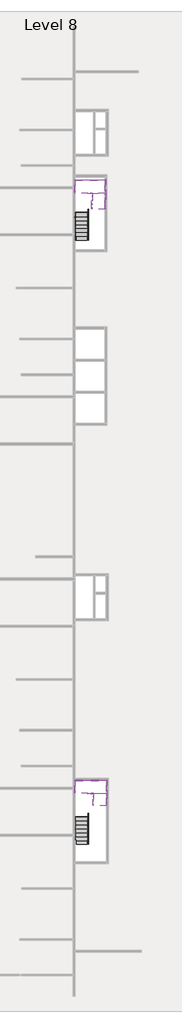
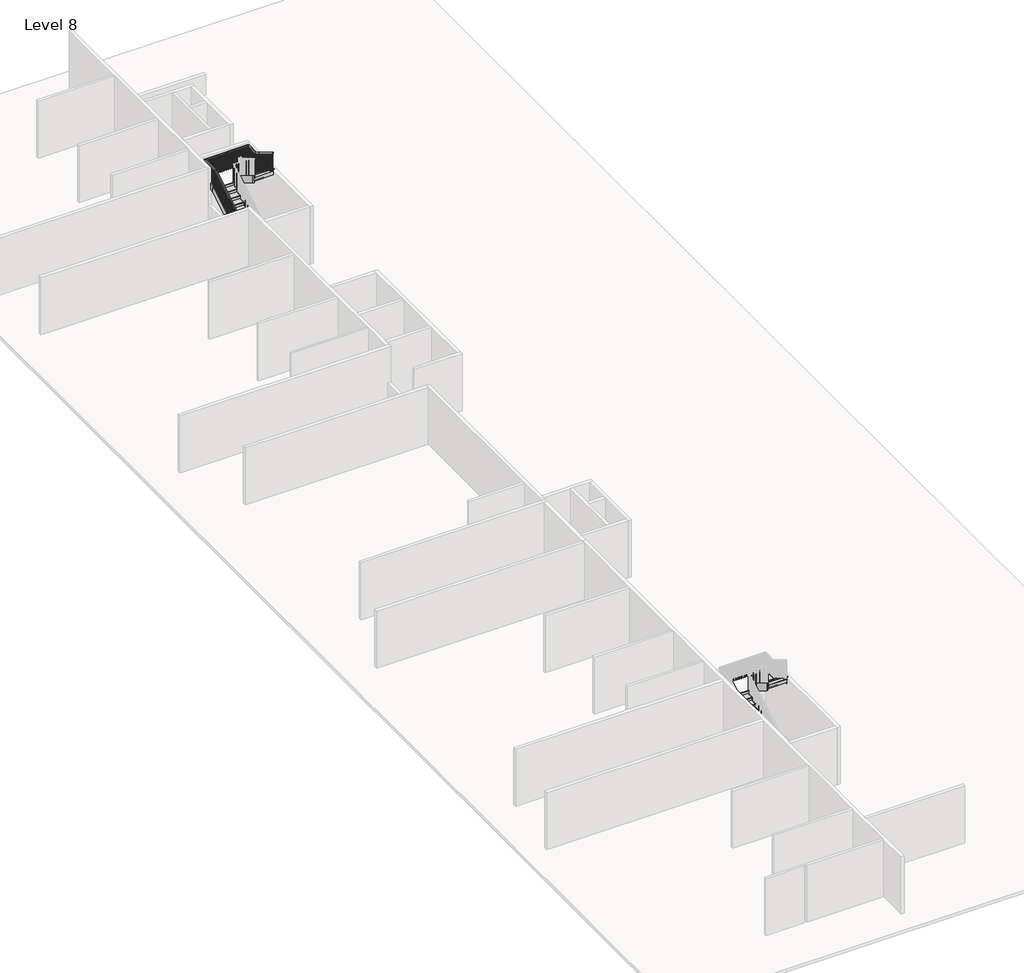
# One storey, part 8 of 8: 16 members, 4 stair flights, 2 slabs, 1 railing.
"""IFC4 building model written with IfcOpenShell, lengths in millimetres."""

from ifc_helpers import new_model, si_unit, frame, origin, place, context, project, spatial, polyline, outline, extrude, faceted_brep, transform, mapped, element, save
from components import non_monolithic_landing_8e40c115, non_monolithic_landing_da8bd63b, stair_flight_80be26fe, stair_flight_738362f5, stair_flight_d970984e, stair_flight_6e3cd39c

model = new_model("IFC4")

# Units and contexts
model_context = context("Model", 3, world=origin())
ifc_project = project(units=[si_unit("LENGTHUNIT", "METRE", prefix="MILLI")], contexts=[model_context])

# Site, building, storey
site = spatial("IfcSite", under=ifc_project)
building = spatial("IfcBuilding", under=site)
storey = spatial("IfcBuildingStorey", under=building, Name="Level 8", Elevation=46570.6172466)

# Members
placement = place(None, origin())
element("IfcMember", 1, ObjectType="Stringer - 2\" Width", at=placement, inside=storey, context=model_context, shape_type="SweptSolid", body=[
    extrude(outline(polyline([(-23154.3851539, 46570.6172466), (-23154.3851539, 46782.7317586), (-19467.0440987, 49017.4839133), (-19381.8896422, 48712.6839133), (-22916.2996422, 46570.6172466), (-23154.3851539, 46570.6172466)])), frame((-3668.2415084, 0.0, 0.0), z_axis=(1.0, 0.0, 0.0), x_axis=(0.0, 1.0, 0.0)), (0.0, 0.0, 1.0), 50.8),
])
element("IfcMember", 2, ObjectType="Stringer - 2\" Width", at=placement, inside=storey, context=model_context, shape_type="SweptSolid", body=[
    extrude(outline(polyline([(-23154.3851539, 46570.6172466), (-23154.3851539, 46782.7317586), (-19572.9851539, 48953.2772131), (-19572.9851539, 48596.8684516), (-22916.2996422, 46570.6172466), (-23154.3851539, 46570.6172466)])), frame((-2703.0415084, 0.0, 0.0), z_axis=(1.0, 0.0, 0.0), x_axis=(0.0, 1.0, 0.0)), (0.0, 0.0, 1.0), 50.8),
])
element("IfcMember", 3, ObjectType="Stringer - 2\" Width", at=placement, inside=storey, context=model_context, shape_type="SweptSolid", body=[
    extrude(outline(polyline([(-19297.9262092, 49017.4839133), (-19383.0806657, 48712.6839133), (-20360.3851539, 49304.9896637), (-20360.3851539, 49661.3984252), (-19297.9262092, 49017.4839133)])), frame((-1382.2415084, 0.0, 0.0), z_axis=(1.0, 0.0, 0.0), x_axis=(0.0, 1.0, 0.0)), (0.0, 0.0, 1.0), 50.8),
])
element("IfcMember", 4, ObjectType="Stringer - 2\" Width", at=placement, inside=storey, context=model_context, shape_type="SweptSolid", body=[
    extrude(outline(polyline([(-19522.1851539, 49153.3984252), (-19522.1851539, 48796.9896637), (-20360.3851539, 49304.9896637), (-20360.3851539, 49661.3984252), (-19522.1851539, 49153.3984252)])), frame((-2347.4415084, 0.0, 0.0), z_axis=(1.0, 0.0, 0.0), x_axis=(0.0, 1.0, 0.0)), (0.0, 0.0, 1.0), 50.8),
])
element("IfcMember", 5, ObjectType="Stringer - 2\" Width", at=placement, inside=storey, context=model_context, shape_type="Brep", body=[
    faceted_brep([(-1382.2415084, -19297.9262092, 49017.4839133), (-1331.4415084, -19297.9262092, 49017.4839133), (-1331.4415084, -18556.9851539, 49017.4839133), (-1382.2415084, -18607.7851539, 49017.4839133), (-1382.2415084, -19383.0806657, 48712.6839133), (-1382.2415084, -18607.7851539, 48712.6839133), (-1331.4415084, -19383.0806657, 48712.6839133), (-1331.4415084, -18556.9851539, 48712.6839133)], [[[0, 1, 2, 3]], [[4, 0, 3, 5]], [[6, 4, 5, 7]], [[1, 6, 7, 2]], [[1, 0, 4, 6]], [[2, 7, 5, 3]]]),
])
element("IfcMember", 6, ObjectType="Stringer - 2\" Width", at=placement, inside=storey, context=model_context, shape_type="SweptSolid", body=[
    extrude(outline(polyline([(-1331.4415084, -18556.9851539), (-1382.2415084, -18607.7851539), (-3617.4415084, -18607.7851539), (-3668.2415084, -18556.9851539), (-1331.4415084, -18556.9851539)])), frame((0.0, 0.0, 48712.6839133), z_axis=(0.0, 0.0, 1.0), x_axis=(1.0, 0.0, 0.0)), (0.0, 0.0, 1.0), 304.8),
])
element("IfcMember", 7, ObjectType="Stringer - 2\" Width", at=placement, inside=storey, context=model_context, shape_type="Brep", body=[
    faceted_brep([(-3617.4415084, -18607.7851539, 49017.4839133), (-3668.2415084, -18556.9851539, 49017.4839133), (-3668.2415084, -19467.0440987, 49017.4839133), (-3617.4415084, -19467.0440987, 49017.4839133), (-3617.4415084, -18607.7851539, 48712.6839133), (-3617.4415084, -19381.8896422, 48712.6839133), (-3668.2415084, -18556.9851539, 48712.6839133), (-3668.2415084, -19381.8896422, 48712.6839133)], [[[0, 1, 2, 3]], [[4, 0, 3, 5]], [[6, 4, 5, 7]], [[1, 6, 7, 2]], [[1, 0, 4, 6]], [[2, 7, 5, 3]]]),
])
element("IfcMember", 8, ObjectType="Stringer - 2\" Width", at=placement, inside=storey, context=model_context, shape_type="SweptSolid", body=[
    extrude(outline(polyline([(-2703.0415084, -19572.9851539), (-2703.0415084, -19522.1851539), (-2347.4415084, -19522.1851539), (-2347.4415084, -19572.9851539), (-2703.0415084, -19572.9851539)])), frame((0.0, 0.0, 48712.6839133), z_axis=(0.0, 0.0, 1.0), x_axis=(1.0, 0.0, 0.0)), (0.0, 0.0, 1.0), 304.8),
])
element("IfcMember", 9, ObjectType="Stringer - 2\" Width", at=placement, inside=storey, context=model_context, shape_type="SweptSolid", body=[
    extrude(outline(polyline([(19841.9216096, 46570.6172466), (19841.9216096, 46782.7317586), (23249.8626649, 48848.1505799), (23335.0171214, 48543.3505799), (20080.0071214, 46570.6172466), (19841.9216096, 46570.6172466)])), frame((-3668.2415084, 0.0, 0.0), z_axis=(1.0, 0.0, 0.0), x_axis=(0.0, 1.0, 0.0)), (0.0, 0.0, 1.0), 50.8),
])
element("IfcMember", 10, ObjectType="Stringer - 2\" Width", at=placement, inside=storey, context=model_context, shape_type="SweptSolid", body=[
    extrude(outline(polyline([(19841.9216096, 46570.6172466), (19841.9216096, 46782.7317586), (23143.9216096, 48783.9438798), (23143.9216096, 48427.5351183), (20080.0071214, 46570.6172466), (19841.9216096, 46570.6172466)])), frame((-2703.0415084, 0.0, 0.0), z_axis=(1.0, 0.0, 0.0), x_axis=(0.0, 1.0, 0.0)), (0.0, 0.0, 1.0), 50.8),
])
element("IfcMember", 11, ObjectType="Stringer - 2\" Width", at=placement, inside=storey, context=model_context, shape_type="SweptSolid", body=[
    extrude(outline(polyline([(23418.9805543, 48848.1505799), (23333.8260978, 48543.3505799), (22077.1216096, 49304.9896637), (22077.1216096, 49661.3984252), (23418.9805543, 48848.1505799)])), frame((-1483.8415084, 0.0, 0.0), z_axis=(1.0, 0.0, 0.0), x_axis=(0.0, 1.0, 0.0)), (0.0, 0.0, 1.0), 50.8),
])
element("IfcMember", 12, ObjectType="Stringer - 2\" Width", at=placement, inside=storey, context=model_context, shape_type="SweptSolid", body=[
    extrude(outline(polyline([(23194.7216096, 48984.0650919), (23194.7216096, 48627.6563304), (22077.1216096, 49304.9896637), (22077.1216096, 49661.3984252), (23194.7216096, 48984.0650919)])), frame((-2449.0415084, 0.0, 0.0), z_axis=(1.0, 0.0, 0.0), x_axis=(0.0, 1.0, 0.0)), (0.0, 0.0, 1.0), 50.8),
])
element("IfcMember", 13, ObjectType="Stringer - 2\" Width", at=placement, inside=storey, context=model_context, shape_type="Brep", body=[
    faceted_brep([(-1483.8415084, 23418.9805543, 48848.1505799), (-1433.0415084, 23418.9805543, 48848.1505799), (-1433.0415084, 24159.9216096, 48848.1505799), (-1483.8415084, 24109.1216096, 48848.1505799), (-1483.8415084, 23333.8260978, 48543.3505799), (-1483.8415084, 24109.1216096, 48543.3505799), (-1433.0415084, 23333.8260978, 48543.3505799), (-1433.0415084, 24159.9216096, 48543.3505799)], [[[0, 1, 2, 3]], [[4, 0, 3, 5]], [[6, 4, 5, 7]], [[1, 6, 7, 2]], [[1, 0, 4, 6]], [[2, 7, 5, 3]]]),
])
element("IfcMember", 14, ObjectType="Stringer - 2\" Width", at=placement, inside=storey, context=model_context, shape_type="SweptSolid", body=[
    extrude(outline(polyline([(-1433.0415084, 24159.9216096), (-1483.8415084, 24109.1216096), (-3617.4415084, 24109.1216096), (-3668.2415084, 24159.9216096), (-1433.0415084, 24159.9216096)])), frame((0.0, 0.0, 48543.3505799), z_axis=(0.0, 0.0, 1.0), x_axis=(1.0, 0.0, 0.0)), (0.0, 0.0, 1.0), 304.8),
])
element("IfcMember", 15, ObjectType="Stringer - 2\" Width", at=placement, inside=storey, context=model_context, shape_type="Brep", body=[
    faceted_brep([(-3617.4415084, 24109.1216096, 48848.1505799), (-3668.2415084, 24159.9216096, 48848.1505799), (-3668.2415084, 23249.8626649, 48848.1505799), (-3617.4415084, 23249.8626649, 48848.1505799), (-3617.4415084, 24109.1216096, 48543.3505799), (-3617.4415084, 23335.0171214, 48543.3505799), (-3668.2415084, 24159.9216096, 48543.3505799), (-3668.2415084, 23335.0171214, 48543.3505799)], [[[0, 1, 2, 3]], [[4, 0, 3, 5]], [[6, 4, 5, 7]], [[1, 6, 7, 2]], [[1, 0, 4, 6]], [[2, 7, 5, 3]]]),
])
element("IfcMember", 16, ObjectType="Stringer - 2\" Width", at=placement, inside=storey, context=model_context, shape_type="SweptSolid", body=[
    extrude(outline(polyline([(-2703.0415084, 23143.9216096), (-2703.0415084, 23194.7216096), (-2449.0415084, 23194.7216096), (-2449.0415084, 23143.9216096), (-2703.0415084, 23143.9216096)])), frame((0.0, 0.0, 48543.3505799), z_axis=(0.0, 0.0, 1.0), x_axis=(1.0, 0.0, 0.0)), (0.0, 0.0, 1.0), 304.8),
])

# Railing
element("IfcRailing", 17, ObjectType="Handrail - Rectangular", at=placement, inside=storey, context=model_context, shape_type="SolidModel", body=[
    faceted_brep([(-3617.4415084, 19841.9216096, 47654.3505799), (-3617.4415084, 19841.9216096, 47594.9491197), (-3566.6415084, 19841.9216096, 47594.9491197), (-3566.6415084, 19841.9216096, 47654.3505799), (-3617.4415084, 23194.7216096, 49686.3505799), (-3617.4415084, 23208.914019, 49635.5505799), (-3566.6415084, 23208.914019, 49635.5505799), (-3566.6415084, 23194.7216096, 49686.3505799), (-3617.4415084, 24109.1216096, 49686.3505799), (-3617.4415084, 24109.1216096, 49635.5505799), (-3566.6415084, 24058.3216096, 49635.5505799), (-3566.6415084, 24058.3216096, 49686.3505799), (-1483.8415084, 24109.1216096, 49686.3505799), (-1483.8415084, 24109.1216096, 49635.5505799), (-1534.6415084, 24058.3216096, 49635.5505799), (-1534.6415084, 24058.3216096, 49686.3505799), (-1483.8415084, 23474.1216096, 49686.3505799), (-1483.8415084, 23459.9292002, 49635.5505799), (-1534.6415084, 23459.9292002, 49635.5505799), (-1534.6415084, 23474.1216096, 49686.3505799), (-1483.8415084, 23194.7216096, 49855.6839133), (-1483.8415084, 23168.3918824, 49812.2398634), (-1534.6415084, 23168.3918824, 49812.2398634), (-1534.6415084, 23194.7216096, 49855.6839133), (-1483.8415084, 22077.1216096, 50533.0172466), (-1534.6415084, 22077.1216096, 50533.0172466), (-1534.6415084, 22077.1216096, 50473.6157863), (-1483.8415084, 22077.1216096, 50473.6157863)], [[[0, 1, 2, 3]], [[1, 0, 4, 5]], [[2, 1, 5, 6]], [[3, 2, 6, 7]], [[0, 3, 7, 4]], [[5, 4, 8, 9]], [[6, 5, 9, 10]], [[7, 6, 10, 11]], [[4, 7, 11, 8]], [[9, 8, 12, 13]], [[10, 9, 13, 14]], [[11, 10, 14, 15]], [[8, 11, 15, 12]], [[13, 12, 16, 17]], [[14, 13, 17, 18]], [[15, 14, 18, 19]], [[12, 15, 19, 16]], [[17, 16, 20, 21]], [[18, 17, 21, 22]], [[19, 18, 22, 23]], [[16, 19, 23, 20]], [[24, 25, 26, 27]], [[21, 20, 24, 27]], [[22, 21, 27, 26]], [[23, 22, 26, 25]], [[20, 23, 25, 24]]]),
    extrude(outline(polyline([(22188.2466096, 50406.2673015), (22188.2466096, 49449.2839133), (22169.1966096, 49449.2839133), (22169.1966096, 50417.812756), (22188.2466096, 50406.2673015)])), frame((-1518.7665084, 0.0, 0.0), z_axis=(1.0, 0.0, 0.0), x_axis=(0.0, 1.0, 0.0)), (0.0, 0.0, 1.0), 19.05),
    extrude(outline(polyline([(22289.8466096, 50344.6915439), (22289.8466096, 49449.2839133), (22270.7966096, 49449.2839133), (22270.7966096, 50356.2369985), (22289.8466096, 50344.6915439)])), frame((-1518.7665084, 0.0, 0.0), z_axis=(1.0, 0.0, 0.0), x_axis=(0.0, 1.0, 0.0)), (0.0, 0.0, 1.0), 19.05),
    extrude(outline(polyline([(22391.4466096, 50283.1157863), (22391.4466096, 49279.9505799), (22372.3966096, 49279.9505799), (22372.3966096, 50294.6612409), (22391.4466096, 50283.1157863)])), frame((-1518.7665084, 0.0, 0.0), z_axis=(1.0, 0.0, 0.0), x_axis=(0.0, 1.0, 0.0)), (0.0, 0.0, 1.0), 19.05),
    extrude(outline(polyline([(22493.0466096, 50221.5400288), (22493.0466096, 49279.9505799), (22473.9966096, 49279.9505799), (22473.9966096, 50233.0854833), (22493.0466096, 50221.5400288)])), frame((-1518.7665084, 0.0, 0.0), z_axis=(1.0, 0.0, 0.0), x_axis=(0.0, 1.0, 0.0)), (0.0, 0.0, 1.0), 19.05),
    extrude(outline(polyline([(22594.6466096, 50159.9642712), (22594.6466096, 49279.9505799), (22575.5966096, 49279.9505799), (22575.5966096, 50171.5097257), (22594.6466096, 50159.9642712)])), frame((-1518.7665084, 0.0, 0.0), z_axis=(1.0, 0.0, 0.0), x_axis=(0.0, 1.0, 0.0)), (0.0, 0.0, 1.0), 19.05),
    extrude(outline(polyline([(22696.2466096, 50098.3885136), (22696.2466096, 49110.6172466), (22677.1966096, 49110.6172466), (22677.1966096, 50109.9339682), (22696.2466096, 50098.3885136)])), frame((-1518.7665084, 0.0, 0.0), z_axis=(1.0, 0.0, 0.0), x_axis=(0.0, 1.0, 0.0)), (0.0, 0.0, 1.0), 19.05),
    extrude(outline(polyline([(22797.8466096, 50036.812756), (22797.8466096, 49110.6172466), (22778.7966096, 49110.6172466), (22778.7966096, 50048.3582106), (22797.8466096, 50036.812756)])), frame((-1518.7665084, 0.0, 0.0), z_axis=(1.0, 0.0, 0.0), x_axis=(0.0, 1.0, 0.0)), (0.0, 0.0, 1.0), 19.05),
    extrude(outline(polyline([(22899.4466096, 49975.2369985), (22899.4466096, 49110.6172466), (22880.3966096, 49110.6172466), (22880.3966096, 49986.782453), (22899.4466096, 49975.2369985)])), frame((-1518.7665084, 0.0, 0.0), z_axis=(1.0, 0.0, 0.0), x_axis=(0.0, 1.0, 0.0)), (0.0, 0.0, 1.0), 19.05),
    extrude(outline(polyline([(23001.0466096, 49913.6612409), (23001.0466096, 48941.2839133), (22981.9966096, 48941.2839133), (22981.9966096, 49925.2066954), (23001.0466096, 49913.6612409)])), frame((-1518.7665084, 0.0, 0.0), z_axis=(1.0, 0.0, 0.0), x_axis=(0.0, 1.0, 0.0)), (0.0, 0.0, 1.0), 19.05),
    extrude(outline(polyline([(23102.6466096, 49852.0854833), (23102.6466096, 48941.2839133), (23083.5966096, 48941.2839133), (23083.5966096, 49863.6309379), (23102.6466096, 49852.0854833)])), frame((-1518.7665084, 0.0, 0.0), z_axis=(1.0, 0.0, 0.0), x_axis=(0.0, 1.0, 0.0)), (0.0, 0.0, 1.0), 19.05),
    extrude(outline(polyline([(23280.4466096, 49744.3279076), (23280.4466096, 48771.9505799), (23261.3966096, 48771.9505799), (23261.3966096, 49755.8733621), (23280.4466096, 49744.3279076)])), frame((-1518.7665084, 0.0, 0.0), z_axis=(1.0, 0.0, 0.0), x_axis=(0.0, 1.0, 0.0)), (0.0, 0.0, 1.0), 19.05),
    extrude(outline(polyline([(23382.0466096, 49682.75215), (23382.0466096, 48771.9505799), (23362.9966096, 48771.9505799), (23362.9966096, 49694.2976045), (23382.0466096, 49682.75215)])), frame((-1518.7665084, 0.0, 0.0), z_axis=(1.0, 0.0, 0.0), x_axis=(0.0, 1.0, 0.0)), (0.0, 0.0, 1.0), 19.05),
    extrude(outline(polyline([(-1499.7165084, 23483.6466096), (-1499.7165084, 23464.5966096), (-1518.7665084, 23464.5966096), (-1518.7665084, 23483.6466096), (-1499.7165084, 23483.6466096)])), frame((0.0, 0.0, 48771.9505799), z_axis=(0.0, 0.0, 1.0), x_axis=(1.0, 0.0, 0.0)), (0.0, 0.0, 1.0), 863.6),
    extrude(outline(polyline([(-1499.7165084, 23585.2466096), (-1499.7165084, 23566.1966096), (-1518.7665084, 23566.1966096), (-1518.7665084, 23585.2466096), (-1499.7165084, 23585.2466096)])), frame((0.0, 0.0, 48771.9505799), z_axis=(0.0, 0.0, 1.0), x_axis=(1.0, 0.0, 0.0)), (0.0, 0.0, 1.0), 863.6),
    extrude(outline(polyline([(-1499.7165084, 23686.8466096), (-1499.7165084, 23667.7966096), (-1518.7665084, 23667.7966096), (-1518.7665084, 23686.8466096), (-1499.7165084, 23686.8466096)])), frame((0.0, 0.0, 48771.9505799), z_axis=(0.0, 0.0, 1.0), x_axis=(1.0, 0.0, 0.0)), (0.0, 0.0, 1.0), 863.6),
    extrude(outline(polyline([(-1499.7165084, 23788.4466096), (-1499.7165084, 23769.3966096), (-1518.7665084, 23769.3966096), (-1518.7665084, 23788.4466096), (-1499.7165084, 23788.4466096)])), frame((0.0, 0.0, 48771.9505799), z_axis=(0.0, 0.0, 1.0), x_axis=(1.0, 0.0, 0.0)), (0.0, 0.0, 1.0), 863.6),
    extrude(outline(polyline([(-1499.7165084, 23890.0466096), (-1499.7165084, 23870.9966096), (-1518.7665084, 23870.9966096), (-1518.7665084, 23890.0466096), (-1499.7165084, 23890.0466096)])), frame((0.0, 0.0, 48771.9505799), z_axis=(0.0, 0.0, 1.0), x_axis=(1.0, 0.0, 0.0)), (0.0, 0.0, 1.0), 863.6),
    extrude(outline(polyline([(-1499.7165084, 23991.6466096), (-1499.7165084, 23972.5966096), (-1518.7665084, 23972.5966096), (-1518.7665084, 23991.6466096), (-1499.7165084, 23991.6466096)])), frame((0.0, 0.0, 48771.9505799), z_axis=(0.0, 0.0, 1.0), x_axis=(1.0, 0.0, 0.0)), (0.0, 0.0, 1.0), 863.6),
    extrude(outline(polyline([(-1569.5665084, 24093.2466096), (-1550.5165084, 24093.2466096), (-1550.5165084, 24074.1966096), (-1569.5665084, 24074.1966096), (-1569.5665084, 24093.2466096)])), frame((0.0, 0.0, 48771.9505799), z_axis=(0.0, 0.0, 1.0), x_axis=(1.0, 0.0, 0.0)), (0.0, 0.0, 1.0), 863.6),
    extrude(outline(polyline([(-1671.1665084, 24093.2466096), (-1652.1165084, 24093.2466096), (-1652.1165084, 24074.1966096), (-1671.1665084, 24074.1966096), (-1671.1665084, 24093.2466096)])), frame((0.0, 0.0, 48771.9505799), z_axis=(0.0, 0.0, 1.0), x_axis=(1.0, 0.0, 0.0)), (0.0, 0.0, 1.0), 863.6),
    extrude(outline(polyline([(-1772.7665084, 24093.2466096), (-1753.7165084, 24093.2466096), (-1753.7165084, 24074.1966096), (-1772.7665084, 24074.1966096), (-1772.7665084, 24093.2466096)])), frame((0.0, 0.0, 48771.9505799), z_axis=(0.0, 0.0, 1.0), x_axis=(1.0, 0.0, 0.0)), (0.0, 0.0, 1.0), 863.6),
    extrude(outline(polyline([(-1874.3665084, 24093.2466096), (-1855.3165084, 24093.2466096), (-1855.3165084, 24074.1966096), (-1874.3665084, 24074.1966096), (-1874.3665084, 24093.2466096)])), frame((0.0, 0.0, 48771.9505799), z_axis=(0.0, 0.0, 1.0), x_axis=(1.0, 0.0, 0.0)), (0.0, 0.0, 1.0), 863.6),
    extrude(outline(polyline([(-1975.9665084, 24093.2466096), (-1956.9165084, 24093.2466096), (-1956.9165084, 24074.1966096), (-1975.9665084, 24074.1966096), (-1975.9665084, 24093.2466096)])), frame((0.0, 0.0, 48771.9505799), z_axis=(0.0, 0.0, 1.0), x_axis=(1.0, 0.0, 0.0)), (0.0, 0.0, 1.0), 863.6),
    extrude(outline(polyline([(-2077.5665084, 24093.2466096), (-2058.5165084, 24093.2466096), (-2058.5165084, 24074.1966096), (-2077.5665084, 24074.1966096), (-2077.5665084, 24093.2466096)])), frame((0.0, 0.0, 48771.9505799), z_axis=(0.0, 0.0, 1.0), x_axis=(1.0, 0.0, 0.0)), (0.0, 0.0, 1.0), 863.6),
    extrude(outline(polyline([(-2179.1665084, 24093.2466096), (-2160.1165084, 24093.2466096), (-2160.1165084, 24074.1966096), (-2179.1665084, 24074.1966096), (-2179.1665084, 24093.2466096)])), frame((0.0, 0.0, 48771.9505799), z_axis=(0.0, 0.0, 1.0), x_axis=(1.0, 0.0, 0.0)), (0.0, 0.0, 1.0), 863.6),
    extrude(outline(polyline([(-2280.7665084, 24093.2466096), (-2261.7165084, 24093.2466096), (-2261.7165084, 24074.1966096), (-2280.7665084, 24074.1966096), (-2280.7665084, 24093.2466096)])), frame((0.0, 0.0, 48771.9505799), z_axis=(0.0, 0.0, 1.0), x_axis=(1.0, 0.0, 0.0)), (0.0, 0.0, 1.0), 863.6),
    extrude(outline(polyline([(-2382.3665084, 24093.2466096), (-2363.3165084, 24093.2466096), (-2363.3165084, 24074.1966096), (-2382.3665084, 24074.1966096), (-2382.3665084, 24093.2466096)])), frame((0.0, 0.0, 48771.9505799), z_axis=(0.0, 0.0, 1.0), x_axis=(1.0, 0.0, 0.0)), (0.0, 0.0, 1.0), 863.6),
    extrude(outline(polyline([(-2483.9665084, 24093.2466096), (-2464.9165084, 24093.2466096), (-2464.9165084, 24074.1966096), (-2483.9665084, 24074.1966096), (-2483.9665084, 24093.2466096)])), frame((0.0, 0.0, 48771.9505799), z_axis=(0.0, 0.0, 1.0), x_axis=(1.0, 0.0, 0.0)), (0.0, 0.0, 1.0), 863.6),
    extrude(outline(polyline([(-2585.5665084, 24093.2466096), (-2566.5165084, 24093.2466096), (-2566.5165084, 24074.1966096), (-2585.5665084, 24074.1966096), (-2585.5665084, 24093.2466096)])), frame((0.0, 0.0, 48771.9505799), z_axis=(0.0, 0.0, 1.0), x_axis=(1.0, 0.0, 0.0)), (0.0, 0.0, 1.0), 863.6),
    extrude(outline(polyline([(-2687.1665084, 24093.2466096), (-2668.1165084, 24093.2466096), (-2668.1165084, 24074.1966096), (-2687.1665084, 24074.1966096), (-2687.1665084, 24093.2466096)])), frame((0.0, 0.0, 48771.9505799), z_axis=(0.0, 0.0, 1.0), x_axis=(1.0, 0.0, 0.0)), (0.0, 0.0, 1.0), 863.6),
    extrude(outline(polyline([(-2788.7665084, 24093.2466096), (-2769.7165084, 24093.2466096), (-2769.7165084, 24074.1966096), (-2788.7665084, 24074.1966096), (-2788.7665084, 24093.2466096)])), frame((0.0, 0.0, 48771.9505799), z_axis=(0.0, 0.0, 1.0), x_axis=(1.0, 0.0, 0.0)), (0.0, 0.0, 1.0), 863.6),
    extrude(outline(polyline([(-2890.3665084, 24093.2466096), (-2871.3165084, 24093.2466096), (-2871.3165084, 24074.1966096), (-2890.3665084, 24074.1966096), (-2890.3665084, 24093.2466096)])), frame((0.0, 0.0, 48771.9505799), z_axis=(0.0, 0.0, 1.0), x_axis=(1.0, 0.0, 0.0)), (0.0, 0.0, 1.0), 863.6),
    extrude(outline(polyline([(-2991.9665084, 24093.2466096), (-2972.9165084, 24093.2466096), (-2972.9165084, 24074.1966096), (-2991.9665084, 24074.1966096), (-2991.9665084, 24093.2466096)])), frame((0.0, 0.0, 48771.9505799), z_axis=(0.0, 0.0, 1.0), x_axis=(1.0, 0.0, 0.0)), (0.0, 0.0, 1.0), 863.6),
    extrude(outline(polyline([(-3093.5665084, 24093.2466096), (-3074.5165084, 24093.2466096), (-3074.5165084, 24074.1966096), (-3093.5665084, 24074.1966096), (-3093.5665084, 24093.2466096)])), frame((0.0, 0.0, 48771.9505799), z_axis=(0.0, 0.0, 1.0), x_axis=(1.0, 0.0, 0.0)), (0.0, 0.0, 1.0), 863.6),
    extrude(outline(polyline([(-3195.1665084, 24093.2466096), (-3176.1165084, 24093.2466096), (-3176.1165084, 24074.1966096), (-3195.1665084, 24074.1966096), (-3195.1665084, 24093.2466096)])), frame((0.0, 0.0, 48771.9505799), z_axis=(0.0, 0.0, 1.0), x_axis=(1.0, 0.0, 0.0)), (0.0, 0.0, 1.0), 863.6),
    extrude(outline(polyline([(-3296.7665084, 24093.2466096), (-3277.7165084, 24093.2466096), (-3277.7165084, 24074.1966096), (-3296.7665084, 24074.1966096), (-3296.7665084, 24093.2466096)])), frame((0.0, 0.0, 48771.9505799), z_axis=(0.0, 0.0, 1.0), x_axis=(1.0, 0.0, 0.0)), (0.0, 0.0, 1.0), 863.6),
    extrude(outline(polyline([(-3398.3665084, 24093.2466096), (-3379.3165084, 24093.2466096), (-3379.3165084, 24074.1966096), (-3398.3665084, 24074.1966096), (-3398.3665084, 24093.2466096)])), frame((0.0, 0.0, 48771.9505799), z_axis=(0.0, 0.0, 1.0), x_axis=(1.0, 0.0, 0.0)), (0.0, 0.0, 1.0), 863.6),
    extrude(outline(polyline([(-3499.9665084, 24093.2466096), (-3480.9165084, 24093.2466096), (-3480.9165084, 24074.1966096), (-3499.9665084, 24074.1966096), (-3499.9665084, 24093.2466096)])), frame((0.0, 0.0, 48771.9505799), z_axis=(0.0, 0.0, 1.0), x_axis=(1.0, 0.0, 0.0)), (0.0, 0.0, 1.0), 863.6),
    extrude(outline(polyline([(-3601.5665084, 23997.9966096), (-3601.5665084, 24017.0466096), (-3582.5165084, 24017.0466096), (-3582.5165084, 23997.9966096), (-3601.5665084, 23997.9966096)])), frame((0.0, 0.0, 48771.9505799), z_axis=(0.0, 0.0, 1.0), x_axis=(1.0, 0.0, 0.0)), (0.0, 0.0, 1.0), 863.6),
    extrude(outline(polyline([(-3601.5665084, 23896.3966096), (-3601.5665084, 23915.4466096), (-3582.5165084, 23915.4466096), (-3582.5165084, 23896.3966096), (-3601.5665084, 23896.3966096)])), frame((0.0, 0.0, 48771.9505799), z_axis=(0.0, 0.0, 1.0), x_axis=(1.0, 0.0, 0.0)), (0.0, 0.0, 1.0), 863.6),
    extrude(outline(polyline([(-3601.5665084, 23794.7966096), (-3601.5665084, 23813.8466096), (-3582.5165084, 23813.8466096), (-3582.5165084, 23794.7966096), (-3601.5665084, 23794.7966096)])), frame((0.0, 0.0, 48771.9505799), z_axis=(0.0, 0.0, 1.0), x_axis=(1.0, 0.0, 0.0)), (0.0, 0.0, 1.0), 863.6),
    extrude(outline(polyline([(-3601.5665084, 23693.1966096), (-3601.5665084, 23712.2466096), (-3582.5165084, 23712.2466096), (-3582.5165084, 23693.1966096), (-3601.5665084, 23693.1966096)])), frame((0.0, 0.0, 48771.9505799), z_axis=(0.0, 0.0, 1.0), x_axis=(1.0, 0.0, 0.0)), (0.0, 0.0, 1.0), 863.6),
    extrude(outline(polyline([(-3601.5665084, 23591.5966096), (-3601.5665084, 23610.6466096), (-3582.5165084, 23610.6466096), (-3582.5165084, 23591.5966096), (-3601.5665084, 23591.5966096)])), frame((0.0, 0.0, 48771.9505799), z_axis=(0.0, 0.0, 1.0), x_axis=(1.0, 0.0, 0.0)), (0.0, 0.0, 1.0), 863.6),
    extrude(outline(polyline([(-3601.5665084, 23489.9966096), (-3601.5665084, 23509.0466096), (-3582.5165084, 23509.0466096), (-3582.5165084, 23489.9966096), (-3601.5665084, 23489.9966096)])), frame((0.0, 0.0, 48771.9505799), z_axis=(0.0, 0.0, 1.0), x_axis=(1.0, 0.0, 0.0)), (0.0, 0.0, 1.0), 863.6),
    extrude(outline(polyline([(-3601.5665084, 23388.3966096), (-3601.5665084, 23407.4466096), (-3582.5165084, 23407.4466096), (-3582.5165084, 23388.3966096), (-3601.5665084, 23388.3966096)])), frame((0.0, 0.0, 48771.9505799), z_axis=(0.0, 0.0, 1.0), x_axis=(1.0, 0.0, 0.0)), (0.0, 0.0, 1.0), 863.6),
    extrude(outline(polyline([(-3601.5665084, 23286.7966096), (-3601.5665084, 23305.8466096), (-3582.5165084, 23305.8466096), (-3582.5165084, 23286.7966096), (-3601.5665084, 23286.7966096)])), frame((0.0, 0.0, 48771.9505799), z_axis=(0.0, 0.0, 1.0), x_axis=(1.0, 0.0, 0.0)), (0.0, 0.0, 1.0), 863.6),
    extrude(outline(polyline([(23102.6466096, 49571.1460894), (23102.6466096, 48602.6172466), (23083.5966096, 48602.6172466), (23083.5966096, 49559.6006348), (23102.6466096, 49571.1460894)])), frame((-3601.5665084, 0.0, 0.0), z_axis=(1.0, 0.0, 0.0), x_axis=(0.0, 1.0, 0.0)), (0.0, 0.0, 1.0), 19.05),
    extrude(outline(polyline([(23001.0466096, 49509.5703318), (23001.0466096, 48602.6172466), (22981.9966096, 48602.6172466), (22981.9966096, 49498.0248773), (23001.0466096, 49509.5703318)])), frame((-3601.5665084, 0.0, 0.0), z_axis=(1.0, 0.0, 0.0), x_axis=(0.0, 1.0, 0.0)), (0.0, 0.0, 1.0), 19.05),
    extrude(outline(polyline([(22899.4466096, 49447.9945742), (22899.4466096, 48433.2839133), (22880.3966096, 48433.2839133), (22880.3966096, 49436.4491197), (22899.4466096, 49447.9945742)])), frame((-3601.5665084, 0.0, 0.0), z_axis=(1.0, 0.0, 0.0), x_axis=(0.0, 1.0, 0.0)), (0.0, 0.0, 1.0), 19.05),
    extrude(outline(polyline([(22797.8466096, 49386.4188166), (22797.8466096, 48433.2839133), (22778.7966096, 48433.2839133), (22778.7966096, 49374.8733621), (22797.8466096, 49386.4188166)])), frame((-3601.5665084, 0.0, 0.0), z_axis=(1.0, 0.0, 0.0), x_axis=(0.0, 1.0, 0.0)), (0.0, 0.0, 1.0), 19.05),
    extrude(outline(polyline([(22696.2466096, 49324.8430591), (22696.2466096, 48433.2839133), (22677.1966096, 48433.2839133), (22677.1966096, 49313.2976045), (22696.2466096, 49324.8430591)])), frame((-3601.5665084, 0.0, 0.0), z_axis=(1.0, 0.0, 0.0), x_axis=(0.0, 1.0, 0.0)), (0.0, 0.0, 1.0), 19.05),
    extrude(outline(polyline([(22594.6466096, 49263.2673015), (22594.6466096, 48263.9505799), (22575.5966096, 48263.9505799), (22575.5966096, 49251.721847), (22594.6466096, 49263.2673015)])), frame((-3601.5665084, 0.0, 0.0), z_axis=(1.0, 0.0, 0.0), x_axis=(0.0, 1.0, 0.0)), (0.0, 0.0, 1.0), 19.05),
    extrude(outline(polyline([(22493.0466096, 49201.6915439), (22493.0466096, 48263.9505799), (22473.9966096, 48263.9505799), (22473.9966096, 49190.1460894), (22493.0466096, 49201.6915439)])), frame((-3601.5665084, 0.0, 0.0), z_axis=(1.0, 0.0, 0.0), x_axis=(0.0, 1.0, 0.0)), (0.0, 0.0, 1.0), 19.05),
    extrude(outline(polyline([(22391.4466096, 49140.1157863), (22391.4466096, 48263.9505799), (22372.3966096, 48263.9505799), (22372.3966096, 49128.5703318), (22391.4466096, 49140.1157863)])), frame((-3601.5665084, 0.0, 0.0), z_axis=(1.0, 0.0, 0.0), x_axis=(0.0, 1.0, 0.0)), (0.0, 0.0, 1.0), 19.05),
    extrude(outline(polyline([(22289.8466096, 49078.5400288), (22289.8466096, 48094.6172466), (22270.7966096, 48094.6172466), (22270.7966096, 49066.9945742), (22289.8466096, 49078.5400288)])), frame((-3601.5665084, 0.0, 0.0), z_axis=(1.0, 0.0, 0.0), x_axis=(0.0, 1.0, 0.0)), (0.0, 0.0, 1.0), 19.05),
    extrude(outline(polyline([(22188.2466096, 49016.9642712), (22188.2466096, 48094.6172466), (22169.1966096, 48094.6172466), (22169.1966096, 49005.4188166), (22188.2466096, 49016.9642712)])), frame((-3601.5665084, 0.0, 0.0), z_axis=(1.0, 0.0, 0.0), x_axis=(0.0, 1.0, 0.0)), (0.0, 0.0, 1.0), 19.05),
    extrude(outline(polyline([(22086.6466096, 48955.3885136), (22086.6466096, 48094.6172466), (22067.5966096, 48094.6172466), (22067.5966096, 48943.8430591), (22086.6466096, 48955.3885136)])), frame((-3601.5665084, 0.0, 0.0), z_axis=(1.0, 0.0, 0.0), x_axis=(0.0, 1.0, 0.0)), (0.0, 0.0, 1.0), 19.05),
    extrude(outline(polyline([(21985.0466096, 48893.812756), (21985.0466096, 47925.2839133), (21965.9966096, 47925.2839133), (21965.9966096, 48882.2673015), (21985.0466096, 48893.812756)])), frame((-3601.5665084, 0.0, 0.0), z_axis=(1.0, 0.0, 0.0), x_axis=(0.0, 1.0, 0.0)), (0.0, 0.0, 1.0), 19.05),
    extrude(outline(polyline([(21883.4466096, 48832.2369985), (21883.4466096, 47925.2839133), (21864.3966096, 47925.2839133), (21864.3966096, 48820.6915439), (21883.4466096, 48832.2369985)])), frame((-3601.5665084, 0.0, 0.0), z_axis=(1.0, 0.0, 0.0), x_axis=(0.0, 1.0, 0.0)), (0.0, 0.0, 1.0), 19.05),
    extrude(outline(polyline([(21781.8466096, 48770.6612409), (21781.8466096, 47755.9505799), (21762.7966096, 47755.9505799), (21762.7966096, 48759.1157863), (21781.8466096, 48770.6612409)])), frame((-3601.5665084, 0.0, 0.0), z_axis=(1.0, 0.0, 0.0), x_axis=(0.0, 1.0, 0.0)), (0.0, 0.0, 1.0), 19.05),
    extrude(outline(polyline([(21680.2466096, 48709.0854833), (21680.2466096, 47755.9505799), (21661.1966096, 47755.9505799), (21661.1966096, 48697.5400288), (21680.2466096, 48709.0854833)])), frame((-3601.5665084, 0.0, 0.0), z_axis=(1.0, 0.0, 0.0), x_axis=(0.0, 1.0, 0.0)), (0.0, 0.0, 1.0), 19.05),
    extrude(outline(polyline([(21578.6466096, 48647.5097257), (21578.6466096, 47755.9505799), (21559.5966096, 47755.9505799), (21559.5966096, 48635.9642712), (21578.6466096, 48647.5097257)])), frame((-3601.5665084, 0.0, 0.0), z_axis=(1.0, 0.0, 0.0), x_axis=(0.0, 1.0, 0.0)), (0.0, 0.0, 1.0), 19.05),
    extrude(outline(polyline([(21477.0466096, 48585.9339682), (21477.0466096, 47586.6172466), (21457.9966096, 47586.6172466), (21457.9966096, 48574.3885136), (21477.0466096, 48585.9339682)])), frame((-3601.5665084, 0.0, 0.0), z_axis=(1.0, 0.0, 0.0), x_axis=(0.0, 1.0, 0.0)), (0.0, 0.0, 1.0), 19.05),
    extrude(outline(polyline([(21375.4466096, 48524.3582106), (21375.4466096, 47586.6172466), (21356.3966096, 47586.6172466), (21356.3966096, 48512.812756), (21375.4466096, 48524.3582106)])), frame((-3601.5665084, 0.0, 0.0), z_axis=(1.0, 0.0, 0.0), x_axis=(0.0, 1.0, 0.0)), (0.0, 0.0, 1.0), 19.05),
    extrude(outline(polyline([(21273.8466096, 48462.782453), (21273.8466096, 47586.6172466), (21254.7966096, 47586.6172466), (21254.7966096, 48451.2369985), (21273.8466096, 48462.782453)])), frame((-3601.5665084, 0.0, 0.0), z_axis=(1.0, 0.0, 0.0), x_axis=(0.0, 1.0, 0.0)), (0.0, 0.0, 1.0), 19.05),
    extrude(outline(polyline([(21172.2466096, 48401.2066954), (21172.2466096, 47417.2839133), (21153.1966096, 47417.2839133), (21153.1966096, 48389.6612409), (21172.2466096, 48401.2066954)])), frame((-3601.5665084, 0.0, 0.0), z_axis=(1.0, 0.0, 0.0), x_axis=(0.0, 1.0, 0.0)), (0.0, 0.0, 1.0), 19.05),
    extrude(outline(polyline([(21070.6466096, 48339.6309379), (21070.6466096, 47417.2839133), (21051.5966096, 47417.2839133), (21051.5966096, 48328.0854833), (21070.6466096, 48339.6309379)])), frame((-3601.5665084, 0.0, 0.0), z_axis=(1.0, 0.0, 0.0), x_axis=(0.0, 1.0, 0.0)), (0.0, 0.0, 1.0), 19.05),
    extrude(outline(polyline([(20969.0466096, 48278.0551803), (20969.0466096, 47417.2839133), (20949.9966096, 47417.2839133), (20949.9966096, 48266.5097257), (20969.0466096, 48278.0551803)])), frame((-3601.5665084, 0.0, 0.0), z_axis=(1.0, 0.0, 0.0), x_axis=(0.0, 1.0, 0.0)), (0.0, 0.0, 1.0), 19.05),
    extrude(outline(polyline([(20867.4466096, 48216.4794227), (20867.4466096, 47247.9505799), (20848.3966096, 47247.9505799), (20848.3966096, 48204.9339682), (20867.4466096, 48216.4794227)])), frame((-3601.5665084, 0.0, 0.0), z_axis=(1.0, 0.0, 0.0), x_axis=(0.0, 1.0, 0.0)), (0.0, 0.0, 1.0), 19.05),
    extrude(outline(polyline([(20765.8466096, 48154.9036651), (20765.8466096, 47247.9505799), (20746.7966096, 47247.9505799), (20746.7966096, 48143.3582106), (20765.8466096, 48154.9036651)])), frame((-3601.5665084, 0.0, 0.0), z_axis=(1.0, 0.0, 0.0), x_axis=(0.0, 1.0, 0.0)), (0.0, 0.0, 1.0), 19.05),
    extrude(outline(polyline([(20664.2466096, 48093.3279076), (20664.2466096, 47078.6172466), (20645.1966096, 47078.6172466), (20645.1966096, 48081.782453), (20664.2466096, 48093.3279076)])), frame((-3601.5665084, 0.0, 0.0), z_axis=(1.0, 0.0, 0.0), x_axis=(0.0, 1.0, 0.0)), (0.0, 0.0, 1.0), 19.05),
    extrude(outline(polyline([(20562.6466096, 48031.75215), (20562.6466096, 47078.6172466), (20543.5966096, 47078.6172466), (20543.5966096, 48020.2066954), (20562.6466096, 48031.75215)])), frame((-3601.5665084, 0.0, 0.0), z_axis=(1.0, 0.0, 0.0), x_axis=(0.0, 1.0, 0.0)), (0.0, 0.0, 1.0), 19.05),
    extrude(outline(polyline([(20461.0466096, 47970.1763924), (20461.0466096, 47078.6172466), (20441.9966096, 47078.6172466), (20441.9966096, 47958.6309379), (20461.0466096, 47970.1763924)])), frame((-3601.5665084, 0.0, 0.0), z_axis=(1.0, 0.0, 0.0), x_axis=(0.0, 1.0, 0.0)), (0.0, 0.0, 1.0), 19.05),
    extrude(outline(polyline([(20359.4466096, 47908.6006348), (20359.4466096, 46909.2839133), (20340.3966096, 46909.2839133), (20340.3966096, 47897.0551803), (20359.4466096, 47908.6006348)])), frame((-3601.5665084, 0.0, 0.0), z_axis=(1.0, 0.0, 0.0), x_axis=(0.0, 1.0, 0.0)), (0.0, 0.0, 1.0), 19.05),
    extrude(outline(polyline([(20257.8466096, 47847.0248773), (20257.8466096, 46909.2839133), (20238.7966096, 46909.2839133), (20238.7966096, 47835.4794227), (20257.8466096, 47847.0248773)])), frame((-3601.5665084, 0.0, 0.0), z_axis=(1.0, 0.0, 0.0), x_axis=(0.0, 1.0, 0.0)), (0.0, 0.0, 1.0), 19.05),
    extrude(outline(polyline([(20156.2466096, 47785.4491197), (20156.2466096, 46909.2839133), (20137.1966096, 46909.2839133), (20137.1966096, 47773.9036651), (20156.2466096, 47785.4491197)])), frame((-3601.5665084, 0.0, 0.0), z_axis=(1.0, 0.0, 0.0), x_axis=(0.0, 1.0, 0.0)), (0.0, 0.0, 1.0), 19.05),
    extrude(outline(polyline([(20054.6466096, 47723.8733621), (20054.6466096, 46739.9505799), (20035.5966096, 46739.9505799), (20035.5966096, 47712.3279076), (20054.6466096, 47723.8733621)])), frame((-3601.5665084, 0.0, 0.0), z_axis=(1.0, 0.0, 0.0), x_axis=(0.0, 1.0, 0.0)), (0.0, 0.0, 1.0), 19.05),
    extrude(outline(polyline([(19953.0466096, 47662.2976045), (19953.0466096, 46739.9505799), (19933.9966096, 46739.9505799), (19933.9966096, 47650.75215), (19953.0466096, 47662.2976045)])), frame((-3601.5665084, 0.0, 0.0), z_axis=(1.0, 0.0, 0.0), x_axis=(0.0, 1.0, 0.0)), (0.0, 0.0, 1.0), 19.05),
    extrude(outline(polyline([(23204.2466096, 49790.5097257), (23204.2466096, 48771.9505799), (23185.1966096, 48771.9505799), (23185.1966096, 49802.0551803), (23204.2466096, 49790.5097257)])), frame((-1518.7665084, 0.0, 0.0), z_axis=(1.0, 0.0, 0.0), x_axis=(0.0, 1.0, 0.0)), (0.0, 0.0, 1.0), 19.05),
    extrude(outline(polyline([(-1518.7665084, 24093.2466096), (-1499.7165084, 24093.2466096), (-1499.7165084, 24074.1966096), (-1518.7665084, 24074.1966096), (-1518.7665084, 24093.2466096)])), frame((0.0, 0.0, 48771.9505799), z_axis=(0.0, 0.0, 1.0), x_axis=(1.0, 0.0, 0.0)), (0.0, 0.0, 1.0), 863.6),
    extrude(outline(polyline([(-3601.5665084, 24074.1966096), (-3601.5665084, 24093.2466096), (-3582.5165084, 24093.2466096), (-3582.5165084, 24074.1966096), (-3601.5665084, 24074.1966096)])), frame((0.0, 0.0, 48771.9505799), z_axis=(0.0, 0.0, 1.0), x_axis=(1.0, 0.0, 0.0)), (0.0, 0.0, 1.0), 863.6),
    extrude(outline(polyline([(23204.2466096, 49632.721847), (23204.2466096, 48771.9505799), (23185.1966096, 48771.9505799), (23185.1966096, 49621.1763924), (23204.2466096, 49632.721847)])), frame((-3601.5665084, 0.0, 0.0), z_axis=(1.0, 0.0, 0.0), x_axis=(0.0, 1.0, 0.0)), (0.0, 0.0, 1.0), 19.05),
    extrude(outline(polyline([(22096.1716096, 50462.0703318), (22096.1716096, 49449.2839133), (22077.1216096, 49449.2839133), (22077.1216096, 50473.6157863), (22096.1716096, 50462.0703318)])), frame((-1518.7665084, 0.0, 0.0), z_axis=(1.0, 0.0, 0.0), x_axis=(0.0, 1.0, 0.0)), (0.0, 0.0, 1.0), 19.05),
    extrude(outline(polyline([(19860.9716096, 47606.4945742), (19860.9716096, 46739.9505799), (19841.9216096, 46739.9505799), (19841.9216096, 47594.9491197), (19860.9716096, 47606.4945742)])), frame((-3601.5665084, 0.0, 0.0), z_axis=(1.0, 0.0, 0.0), x_axis=(0.0, 1.0, 0.0)), (0.0, 0.0, 1.0), 19.05),
])

# Slabs
non_monolithic_landing_shape = non_monolithic_landing_8e40c115(model_context)
element("IfcSlab", 18, ObjectType="Non-Monolithic Landing", at=placement, inside=storey, context=model_context, shape_type="MappedRepresentation", body=[
    mapped(non_monolithic_landing_shape, transform((0.0, 0.0, 0.0), x_axis=(1.0, 0.0, 0.0), y_axis=(0.0, 1.0, 0.0), z_axis=(0.0, 0.0, 1.0))),
])
non_monolithic_landing_2_shape = non_monolithic_landing_da8bd63b(model_context)
element("IfcSlab", 19, ObjectType="Non-Monolithic Landing", at=placement, inside=storey, context=model_context, shape_type="MappedRepresentation", body=[
    mapped(non_monolithic_landing_2_shape, transform((0.0, 0.0, 0.0), x_axis=(1.0, 0.0, 0.0), y_axis=(0.0, 1.0, 0.0), z_axis=(0.0, 0.0, 1.0))),
])

# Stair flights
stair_flight_shape = stair_flight_80be26fe(model_context)
element("IfcStairFlight", 20, ObjectType="2\" Tread 1\" Nosing 1/4\" Riser", at=placement, inside=storey, context=model_context, shape_type="MappedRepresentation", body=[
    mapped(stair_flight_shape, transform((0.0, 0.0, 0.0), x_axis=(1.0, 0.0, 0.0), y_axis=(0.0, 1.0, 0.0), z_axis=(0.0, 0.0, 1.0))),
])
stair_flight_2_shape = stair_flight_738362f5(model_context)
element("IfcStairFlight", 21, ObjectType="2\" Tread 1\" Nosing 1/4\" Riser", at=placement, inside=storey, context=model_context, shape_type="MappedRepresentation", body=[
    mapped(stair_flight_2_shape, transform((0.0, 0.0, 0.0), x_axis=(1.0, 0.0, 0.0), y_axis=(0.0, 1.0, 0.0), z_axis=(0.0, 0.0, 1.0))),
])
stair_flight_3_shape = stair_flight_d970984e(model_context)
element("IfcStairFlight", 22, ObjectType="2\" Tread 1\" Nosing 1/4\" Riser", at=placement, inside=storey, context=model_context, shape_type="MappedRepresentation", body=[
    mapped(stair_flight_3_shape, transform((0.0, 0.0, 0.0), x_axis=(1.0, 0.0, 0.0), y_axis=(0.0, 1.0, 0.0), z_axis=(0.0, 0.0, 1.0))),
])
stair_flight_4_shape = stair_flight_6e3cd39c(model_context)
element("IfcStairFlight", 23, ObjectType="2\" Tread 1\" Nosing 1/4\" Riser", at=placement, inside=storey, context=model_context, shape_type="MappedRepresentation", body=[
    mapped(stair_flight_4_shape, transform((0.0, 0.0, 0.0), x_axis=(1.0, 0.0, 0.0), y_axis=(0.0, 1.0, 0.0), z_axis=(0.0, 0.0, 1.0))),
])

save(model, "model.ifc")

# Revit data of these elements
# Type "Handrail - Rectangular"
#   Assembly Code = "C2010400"
#   built-in parameter 1008612 = 0.0416667 (stored number, unit not read)
#   built-in parameter 1008611 = 0.0416667 (stored number, unit not read)
#   built-in parameter 1008609 = 0.333333 (stored number, unit not read)
#   built-in parameter 1008604 = 0.166667 (stored number, unit not read)
#   built-in parameter 1008603 = 0.166667 (stored number, unit not read)
#   Railing Height = 3' - 0"
#   built-in parameter 1008630 = 2
#   built-in parameter 1008610 = 2
#   built-in parameter 1008618 = Baluster - Square : 3/4"
# Elements 1, 2, 3, 4, 5, 6, 7, 8, 9, 10, 11, 12, 13, 14, 15, 16 (IfcMember, "Stringer - 2\" Width")
#   Phase Created = New Construction
# Element 17 (IfcRailing, "Handrail - Rectangular")
#   Phase Created = New Construction
# Elements 18, 19 (IfcSlab, "Non-Monolithic Landing")
#   Phase Created = New Construction
# Elements 20, 21, 22, 23 (IfcStairFlight, "2\" Tread 1\" Nosing 1/4\" Riser")
#   Phase Created = New Construction
